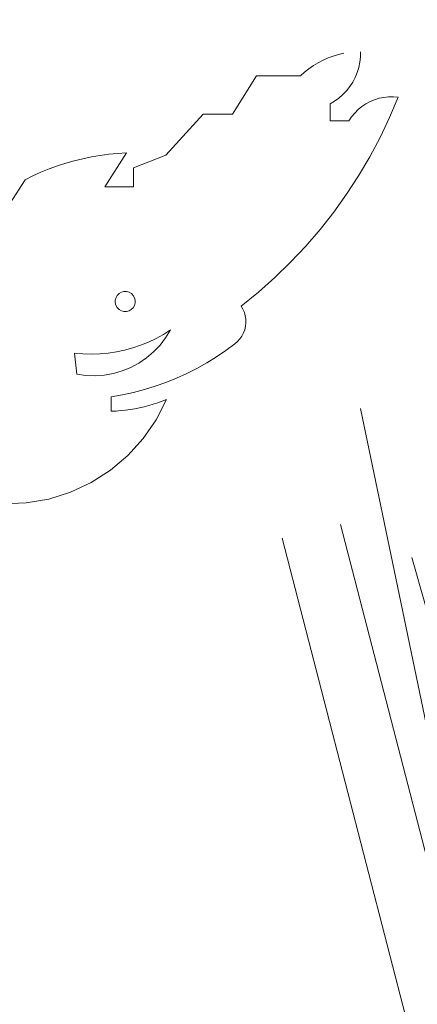
# Model space of a CAD drawing. Units: millimetres. Extents: x 7894 to 8038, y 6851 to 6951.
# Tile 34 of 49: x 7964.635 to 7965.741, y 6925.713 to 6928.453. Entities that reach past the tile are written whole.
import ezdxf

# ---------------------------------------------------------------- set-up
doc = ezdxf.new("R2010")
doc.units = ezdxf.units.MM
doc.layers.add('A-ANNO-DIMS', color=2, linetype='Continuous', lineweight=18)
doc.layers.add('A-FURN-ACCS', color=8, linetype='Continuous', lineweight=13)
doc.styles.get("Standard").update_dxf_attribs({"font": 'arial.ttf'})
doc.dimstyles.new('ISO-25', dxfattribs={"dimtxt": 1, "dimasz": 1, "dimexe": 1.25, "dimexo": 0.625, "dimtad": 1, "dimdec": 0, "dimlunit": 4, "dimtxsty": 'Standard', "dimcen": 2.5, "dimclrt": 1, "dimadec": 0, "dimazin": 0, "dimtfac": 1, "dimtdec": 0, "dimtmove": 0, "dimatfit": 3, "dimfxl": 1, "dimarcsym": 0})

# ---------------------------------------------------------------- blocks, each defined once
blk = doc.blocks.new('DISPLAY-LEAF-FINIAL-Z2_152')
for p, q in [((2.565, 3.5085, 2.1518), (2.5649, 3.4937, 2.1518)), ((2.4472, 3.4779, 2.1518), (2.4609, 3.4849, 2.1518)), ((2.4609, 3.4849, 2.1518), (2.4749, 3.4911, 2.1518)), ((2.4749, 3.4911, 2.1518), (2.4894, 3.4964, 2.1518)), ((2.4894, 3.4964, 2.1518), (2.5041, 3.5007, 2.1518)), ((2.5041, 3.5007, 2.1518), (2.5191, 3.5041, 2.1518)), ((2.5649, 3.4937, 2.1518), (2.5634, 3.479, 2.1518)), ((2.4094, 3.4516, 2.1518), (2.4214, 3.4612, 2.1518)), ((2.4214, 3.4612, 2.1518), (2.4341, 3.4699, 2.1518)), ((2.4341, 3.4699, 2.1518), (2.4472, 3.4779, 2.1518)), ((2.5605, 3.4646, 2.1518), (2.5562, 3.4504, 2.1518)), ((2.5634, 3.479, 2.1518), (2.5605, 3.4646, 2.1518)), ((2.2094, 3.3343, 2.1518), (2.2756, 3.4413, 2.1518)), ((2.2756, 3.4413, 2.1518), (2.3979, 3.4413, 2.1518)), ((2.3979, 3.4413, 2.1518), (2.4094, 3.4516, 2.1518)), ((2.5507, 3.4368, 2.1518), (2.5438, 3.4237, 2.1518)), ((2.5562, 3.4504, 2.1518), (2.5507, 3.4368, 2.1518)), ((2.5266, 3.3997, 2.1518), (2.5164, 3.3891, 2.1518)), ((2.5358, 3.4113, 2.1518), (2.5266, 3.3997, 2.1518)), ((2.5438, 3.4237, 2.1518), (2.5358, 3.4113, 2.1518)), ((2.4932, 3.3709, 2.1518), (2.4804, 3.3636, 2.1518)), ((2.5052, 3.3794, 2.1518), (2.4932, 3.3709, 2.1518)), ((2.5164, 3.3891, 2.1518), (2.5052, 3.3794, 2.1518)), ((2.5917, 3.3696, 2.1518), (2.604, 3.3748, 2.1518)), ((2.604, 3.3748, 2.1518), (2.6168, 3.3788, 2.1518)), ((2.6168, 3.3788, 2.1518), (2.63, 3.3815, 2.1518)), ((2.63, 3.3815, 2.1518), (2.6433, 3.3829, 2.1518)), ((2.6433, 3.3829, 2.1518), (2.6567, 3.3831, 2.1518)), ((2.6701, 3.3819, 2.1518), (2.6462, 3.3254, 2.1518)), ((2.6567, 3.3831, 2.1518), (2.6701, 3.3819, 2.1518)), ((2.4804, 3.3636, 2.1518), (2.4804, 3.3164, 2.1518)), ((2.5489, 3.3378, 2.1518), (2.5584, 3.3473, 2.1518)), ((2.5584, 3.3473, 2.1518), (2.5687, 3.3558, 2.1518)), ((2.5687, 3.3558, 2.1518), (2.5799, 3.3633, 2.1518)), ((2.5799, 3.3633, 2.1518), (2.5917, 3.3696, 2.1518)), ((2.0233, 3.2209, 2.1518), (2.1272, 3.3343, 2.1518)), ((2.1272, 3.3343, 2.1518), (2.2094, 3.3343, 2.1518)), ((2.4804, 3.3164, 2.1518), (2.5329, 3.3164, 2.1518)), ((2.5329, 3.3164, 2.1518), (2.5403, 3.3275, 2.1518)), ((2.5403, 3.3275, 2.1518), (2.5489, 3.3378, 2.1518)), ((2.6462, 3.3254, 2.1518), (2.6199, 3.27, 2.1518)), ((2.6199, 3.27, 2.1518), (2.5912, 3.2159, 2.1518)), ((1.7688, 3.2049, 2.1518), (1.7926, 3.2108, 2.1518)), ((1.7926, 3.2108, 2.1518), (1.8166, 3.2158, 2.1518)), ((1.8166, 3.2158, 2.1518), (1.8408, 3.2199, 2.1518)), ((1.8408, 3.2199, 2.1518), (1.8651, 3.2232, 2.1518)), ((1.9139, 3.2271, 2.1518), (1.8536, 3.1329, 2.1518)), ((1.8651, 3.2232, 2.1518), (1.8895, 3.2256, 2.1518)), ((1.8895, 3.2256, 2.1518), (1.9139, 3.2271, 2.1518)), ((1.934, 3.1854, 2.1518), (2.0233, 3.2209, 2.1518)), ((2.5912, 3.2159, 2.1518), (2.56, 3.1631, 2.1518)), ((1.6762, 3.1731, 2.1518), (1.6989, 3.1823, 2.1518)), ((1.6989, 3.1823, 2.1518), (1.7219, 3.1906, 2.1518)), ((1.7219, 3.1906, 2.1518), (1.7452, 3.1982, 2.1518)), ((1.7452, 3.1982, 2.1518), (1.7688, 3.2049, 2.1518)), ((1.934, 3.1329, 2.1518), (1.934, 3.1854, 2.1518)), ((1.5498, 3.0242, 2.1518), (1.6318, 3.1522, 2.1518)), ((1.6318, 3.1522, 2.1518), (1.6538, 3.163, 2.1518)), ((1.6538, 3.163, 2.1518), (1.6762, 3.1731, 2.1518)), ((2.56, 3.1631, 2.1518), (2.5265, 3.1117, 2.1518)), ((1.8536, 3.1329, 2.1518), (1.934, 3.1329, 2.1518)), ((2.5265, 3.1117, 2.1518), (2.4908, 3.0619, 2.1518)), ((2.4908, 3.0619, 2.1518), (2.4529, 3.0137, 2.1518)), ((2.4529, 3.0137, 2.1518), (2.4129, 2.9672, 2.1518)), ((2.4129, 2.9672, 2.1518), (2.3708, 2.9226, 2.1518)), ((2.3708, 2.9226, 2.1518), (2.3268, 2.8799, 2.1518)), ((2.3268, 2.8799, 2.1518), (2.2809, 2.8392, 2.1518)), ((1.8829, 2.8172, 2.1518), (1.8849, 2.8243, 2.1518)), ((1.8849, 2.8243, 2.1518), (1.8885, 2.8306, 2.1518)), ((1.8885, 2.8306, 2.1518), (1.8937, 2.8357, 2.1518)), ((1.8937, 2.8357, 2.1518), (1.9001, 2.8393, 2.1518)), ((1.9001, 2.8393, 2.1518), (1.9071, 2.8412, 2.1518)), ((1.9071, 2.8412, 2.1518), (1.9144, 2.8411, 2.1518)), ((1.9144, 2.8411, 2.1518), (1.9215, 2.8392, 2.1518)), ((1.9215, 2.8392, 2.1518), (1.9278, 2.8355, 2.1518)), ((1.9278, 2.8355, 2.1518), (1.9329, 2.8304, 2.1518)), ((1.9329, 2.8304, 2.1518), (1.9365, 2.824, 2.1518)), ((1.9365, 2.824, 2.1518), (1.9384, 2.817, 2.1518)), ((2.2809, 2.8392, 2.1518), (2.2333, 2.8006, 2.1518)), ((1.8829, 2.8099, 2.1518), (1.8829, 2.8172, 2.1518)), ((1.8847, 2.8029, 2.1518), (1.8829, 2.8099, 2.1518)), ((1.8884, 2.7965, 2.1518), (1.8847, 2.8029, 2.1518)), ((1.8935, 2.7913, 2.1518), (1.8884, 2.7965, 2.1518)), ((1.9327, 2.7963, 2.1518), (1.9275, 2.7912, 2.1518)), ((1.9364, 2.8026, 2.1518), (1.9327, 2.7963, 2.1518)), ((1.9383, 2.8097, 2.1518), (1.9364, 2.8026, 2.1518)), ((1.9384, 2.817, 2.1518), (1.9383, 2.8097, 2.1518)), ((2.2333, 2.8006, 2.1518), (2.2382, 2.7921, 2.1518)), ((1.8998, 2.7877, 2.1518), (1.8935, 2.7913, 2.1518)), ((1.9068, 2.7857, 2.1518), (1.8998, 2.7877, 2.1518)), ((1.9141, 2.7857, 2.1518), (1.9068, 2.7857, 2.1518)), ((1.9212, 2.7876, 2.1518), (1.9141, 2.7857, 2.1518)), ((1.9275, 2.7912, 2.1518), (1.9212, 2.7876, 2.1518)), ((2.2382, 2.7921, 2.1518), (2.242, 2.7831, 2.1518)), ((2.242, 2.7831, 2.1518), (2.2446, 2.7737, 2.1518)), ((2.2446, 2.7737, 2.1518), (2.246, 2.7641, 2.1518)), ((2.2452, 2.7446, 2.1518), (2.243, 2.7351, 2.1518)), ((2.2462, 2.7543, 2.1518), (2.2452, 2.7446, 2.1518)), ((2.246, 2.7641, 2.1518), (2.2462, 2.7543, 2.1518)), ((2.0167, 2.7218, 2.1518), (1.9962, 2.7106, 2.1518)), ((2.023, 2.7124, 2.1518), (2.0073, 2.692, 2.1518)), ((2.0364, 2.7343, 2.1518), (2.0167, 2.7218, 2.1518)), ((2.0364, 2.7343, 2.1518), (2.023, 2.7124, 2.1518)), ((2.2352, 2.7172, 2.1518), (2.2296, 2.7092, 2.1518)), ((2.2396, 2.7259, 2.1518), (2.2352, 2.7172, 2.1518)), ((2.243, 2.7351, 2.1518), (2.2396, 2.7259, 2.1518)), ((1.9535, 2.6918, 2.1518), (1.9314, 2.6843, 2.1518)), ((1.9751, 2.7005, 2.1518), (1.9535, 2.6918, 2.1518)), ((1.9962, 2.7106, 2.1518), (1.9751, 2.7005, 2.1518)), ((2.0073, 2.692, 2.1518), (1.9895, 2.6734, 2.1518)), ((2.2158, 2.6954, 2.1518), (2.1904, 2.6768, 2.1518)), ((2.2231, 2.7019, 2.1518), (2.2158, 2.6954, 2.1518)), ((2.2296, 2.7092, 2.1518), (2.2231, 2.7019, 2.1518)), ((1.793, 2.6675, 2.1518), (1.7698, 2.6695, 2.1518)), ((1.7698, 2.6695, 2.1518), (1.7755, 2.6114, 2.1518)), ((1.8164, 2.6669, 2.1518), (1.793, 2.6675, 2.1518)), ((1.8397, 2.6677, 2.1518), (1.8164, 2.6669, 2.1518)), ((1.8629, 2.6698, 2.1518), (1.8397, 2.6677, 2.1518)), ((1.886, 2.6733, 2.1518), (1.8629, 2.6698, 2.1518)), ((1.9089, 2.6781, 2.1518), (1.886, 2.6733, 2.1518)), ((1.9314, 2.6843, 2.1518), (1.9089, 2.6781, 2.1518)), ((1.9895, 2.6734, 2.1518), (1.9699, 2.6568, 2.1518)), ((2.1643, 2.6592, 2.1518), (2.1374, 2.6427, 2.1518)), ((2.1904, 2.6768, 2.1518), (2.1643, 2.6592, 2.1518)), ((1.9261, 2.6302, 2.1518), (1.9023, 2.6205, 2.1518)), ((1.9487, 2.6423, 2.1518), (1.9261, 2.6302, 2.1518)), ((1.9699, 2.6568, 2.1518), (1.9487, 2.6423, 2.1518)), ((2.1374, 2.6427, 2.1518), (2.1099, 2.6273, 2.1518)), ((1.8009, 2.6079, 2.1518), (1.7755, 2.6114, 2.1518)), ((1.8266, 2.607, 2.1518), (1.8009, 2.6079, 2.1518)), ((1.8523, 2.6088, 2.1518), (1.8266, 2.607, 2.1518)), ((1.8776, 2.6133, 2.1518), (1.8523, 2.6088, 2.1518)), ((1.9023, 2.6205, 2.1518), (1.8776, 2.6133, 2.1518)), ((2.0818, 2.6132, 2.1518), (2.0531, 2.6002, 2.1518)), ((2.1099, 2.6273, 2.1518), (2.0818, 2.6132, 2.1518)), ((1.9942, 2.5779, 2.1518), (1.9641, 2.5686, 2.1518)), ((2.0239, 2.5884, 2.1518), (1.9942, 2.5779, 2.1518)), ((2.0531, 2.6002, 2.1518), (2.0239, 2.5884, 2.1518)), ((1.9029, 2.5539, 2.1518), (1.8718, 2.5484, 2.1518)), ((1.8718, 2.5484, 2.1518), (1.8718, 2.5082, 2.1518)), ((1.9336, 2.5606, 2.1518), (1.9029, 2.5539, 2.1518)), ((1.9641, 2.5686, 2.1518), (1.9336, 2.5606, 2.1518)), ((1.9502, 2.5177, 2.1518), (1.9631, 2.5206, 2.1518)), ((1.9631, 2.5206, 2.1518), (1.9758, 2.5239, 2.1518)), ((1.9758, 2.5239, 2.1518), (1.9885, 2.5276, 2.1518)), ((1.9885, 2.5276, 2.1518), (2.001, 2.5317, 2.1518)), ((2.0257, 2.5409, 2.1518), (1.9968, 2.4843, 2.1518)), ((2.001, 2.5317, 2.1518), (2.0134, 2.5361, 2.1518)), ((2.0134, 2.5361, 2.1518), (2.0257, 2.5409, 2.1518)), ((1.8718, 2.5082, 2.1518), (1.885, 2.5088, 2.1518)), ((1.885, 2.5088, 2.1518), (1.8981, 2.5098, 2.1518)), ((1.8981, 2.5098, 2.1518), (1.9112, 2.5112, 2.1518)), ((1.9112, 2.5112, 2.1518), (1.9243, 2.513, 2.1518)), ((1.9243, 2.513, 2.1518), (1.9373, 2.5152, 2.1518)), ((1.9373, 2.5152, 2.1518), (1.9502, 2.5177, 2.1518)), ((1.9968, 2.4843, 2.1518), (1.9607, 2.4321, 2.1518)), ((1.9607, 2.4321, 2.1518), (1.918, 2.3851, 2.1518)), ((1.918, 2.3851, 2.1518), (1.8695, 2.3441, 2.1518)), ((1.8695, 2.3441, 2.1518), (1.8161, 2.3099, 2.1518)), ((1.8161, 2.3099, 2.1518), (1.7585, 2.283, 2.1518)), ((1.7585, 2.283, 2.1518), (1.698, 2.2639, 2.1518)), ((1.6354, 2.2529, 2.1518), (1.572, 2.2503, 2.1518)), ((1.698, 2.2639, 2.1518), (1.6354, 2.2529, 2.1518))]:
    blk.add_line(p, q)
blk = doc.blocks.new('DISPLAY-REED-SPRAY')
for p, q in [((1.5483, 0.9938), (1.529, 1.9891)), ((1.7657, 1.0095), (1.7415, 1.9798)), ((0.5154, 1.5733), (0.4354, 1.9715)), ((0.2181, 1.9336), (0.4198, 0.9626)), ((1.7698, 0.9258), (1.8607, 1.8783)), ((1.0617, 0.8114), (0.9453, 1.7069)), ((0.8459, 0.7666), (0.7293, 1.6887)), ((0.5782, 0.0032), (0.1619, 1.6106)), ((1.9375, 0.0029), (2.2747, 1.6026)), ((0, 1.5725), (0.4056, 0.0011)), ((0.9346, 0.1034), (0.5185, 1.5674)), ((2.1079, 0.0011), (2.44, 1.5729)), ((0.7924, 0), (0.3606, 1.5186)), ((1.5597, 0.991), (1.5609, 0.9349)), ((1.753, 0.8924), (1.7508, 0.9993)), ((0.6196, 0.0033), (0.4281, 0.9603)), ((1.5603, 0.9272), (1.5609, 0.9349)), ((1.4766, 0.0028), (1.5603, 0.9272)), ((1.5603, 0.9272), (1.5804, 0.0032)), ((1.753, 0.8924), (1.7551, 0.9145)), ((1.7713, 0.0032), (1.753, 0.8924)), ((1.1386, 0.003), (1.042, 0.8085)), ((0.9346, 0.1034), (0.8517, 0.7803)), ((0.9634, 0.002), (0.9346, 0.1034))]:
    blk.add_line(p, q)
blk = doc.blocks.new('*D23')
at = {"layer": 'A-ANNO-DIMS', "color": 0, "lineweight": -2, "transparency": 16777216}
for p, q in [((7940.0888, 6907.098), (7940.0888, 6947.7928)), ((7971.9356, 6928.989), (7971.9356, 6947.7928)), ((7941.0888, 6946.5428), (7970.9356, 6946.5428))]:
    blk.add_line(p, q, dxfattribs=at)
at = {"layer": 'A-ANNO-DIMS', "color": 0, "transparency": 16777216}
for points in [[(7941.0888, 6946.7095), (7941.0888, 6946.3762), (7940.0888, 6946.5428)], [(7970.9356, 6946.7095), (7970.9356, 6946.3762), (7971.9356, 6946.5428)]]:
    blk.add_solid(points, dxfattribs=at)
at = {"layer": 'Defpoints', "color": 0, "transparency": 16777216}
for p in [(7971.9356, 6946.5428), (7971.9356, 6928.364), (7940.0888, 6906.473)]:
    blk.add_point(p, dxfattribs=at)
at = {"layer": 'A-ANNO-DIMS', "color": 1, "transparency": 16777216, "insert": (7956.0122, 6947.6784), "char_height": 1, "attachment_point": 5}
blk.add_mtext('2\'-8"', dxfattribs=at)
blk = doc.blocks.new('*D28')
at = {"layer": 'A-ANNO-DIMS', "color": 0, "lineweight": -2, "transparency": 16777216}
for p, q in [((7960.8854, 6936.8804), (7975.2272, 6936.8804)), ((7973.9772, 6935.8804), (7973.9772, 6923.6283)), ((7971.8421, 6922.6283), (7975.2272, 6922.6283))]:
    blk.add_line(p, q, dxfattribs=at)
at = {"layer": 'A-ANNO-DIMS', "color": 0, "transparency": 16777216}
for points in [[(7973.8105, 6935.8804), (7974.1439, 6935.8804), (7973.9772, 6936.8804)], [(7973.8105, 6923.6283), (7974.1439, 6923.6283), (7973.9772, 6922.6283)]]:
    blk.add_solid(points, dxfattribs=at)
at = {"layer": 'Defpoints', "color": 0, "transparency": 16777216}
for p in [(7960.2604, 6936.8804), (7971.2171, 6922.6283), (7973.9772, 6922.6283)]:
    blk.add_point(p, dxfattribs=at)
at = {"layer": 'A-ANNO-DIMS', "color": 1, "transparency": 16777216, "insert": (7972.8351, 6929.7543), "char_height": 1, "attachment_point": 5, "rotation": 90}
blk.add_mtext('1\'-2 1/2"', dxfattribs=at)
blk = doc.blocks.new('*D31')
at = {"layer": 'A-ANNO-DIMS', "color": 0, "lineweight": -2, "transparency": 16777216}
for p, q in [((7973.9772, 6921.7198), (7973.9772, 6926.628)), ((7949.8107, 6920.7198), (7975.2272, 6920.7198)), ((7973.9772, 6918.7198), (7973.9772, 6920.7198)), ((7950.9654, 6918.7198), (7975.2272, 6918.7198)), ((7973.9772, 6917.7198), (7973.9772, 6916.7198))]:
    blk.add_line(p, q, dxfattribs=at)
at = {"layer": 'A-ANNO-DIMS', "color": 0, "transparency": 16777216}
for points in [[(7973.8105, 6921.7198), (7974.1439, 6921.7198), (7973.9772, 6920.7198)], [(7973.8105, 6917.7198), (7974.1439, 6917.7198), (7973.9772, 6918.7198)]]:
    blk.add_solid(points, dxfattribs=at)
at = {"layer": 'Defpoints', "color": 0, "transparency": 16777216}
for p in [(7949.1857, 6920.7198), (7973.9772, 6920.7198), (7950.3404, 6918.7198)]:
    blk.add_point(p, dxfattribs=at)
at = {"layer": 'A-ANNO-DIMS', "color": 1, "transparency": 16777216, "insert": (7972.8416, 6924.6739), "char_height": 1, "attachment_point": 5, "rotation": 90}
blk.add_mtext('0\'-2"', dxfattribs=at)

msp = doc.modelspace()

# ---------------------------------------------------------------- block references
at = {"layer": 'A-FURN-ACCS'}
for name, p in [('DISPLAY-LEAF-FINIAL-Z2_152', (7963.0178, 6924.8555)), ('DISPLAY-REED-SPRAY', (7965.365, 6925.4377))]:
    msp.add_blockref(name, p, dxfattribs=at)

# ---------------------------------------------------------------- dimensions: what is measured, and where the dimension line sits
at = {"layer": 'A-ANNO-DIMS'}
dim = msp.add_linear_dim(base=(7971.9356, 6946.5428), p1=(7940.0888, 6906.473), p2=(7971.9356, 6928.364), dimstyle='ISO-25', override={"dimdec": 1, "dimlfac": 1, "dimrnd": 0, "dimzin": 1, "dimdsep": 46, "dimlunit": 4, "dimfrac": 2}, dxfattribs=at)
dim.commit()
dim.dimension.update_dxf_attribs({"geometry": '*D23', "text_midpoint": (7956.0122, 6947.6784)})
for base, p1, p2, picture, middle in [((7973.9772, 6922.6283), (7960.2604, 6936.8804), (7971.2171, 6922.6283), '*D28', (7972.8351, 6929.7543)), ((7973.9772, 6920.7198), (7950.3404, 6918.7198), (7949.1857, 6920.7198), '*D31', (7972.8416, 6924.6739))]:
    dim = msp.add_linear_dim(base=base, p1=p1, p2=p2, angle=90, dimstyle='ISO-25', override={"dimdec": 1, "dimlfac": 1, "dimrnd": 0, "dimzin": 1, "dimdsep": 46, "dimlunit": 4, "dimfrac": 2}, dxfattribs=at)
    dim.commit()
    dim.dimension.update_dxf_attribs({"geometry": picture, "text_midpoint": middle})

doc.saveas('drawing.dxf')
